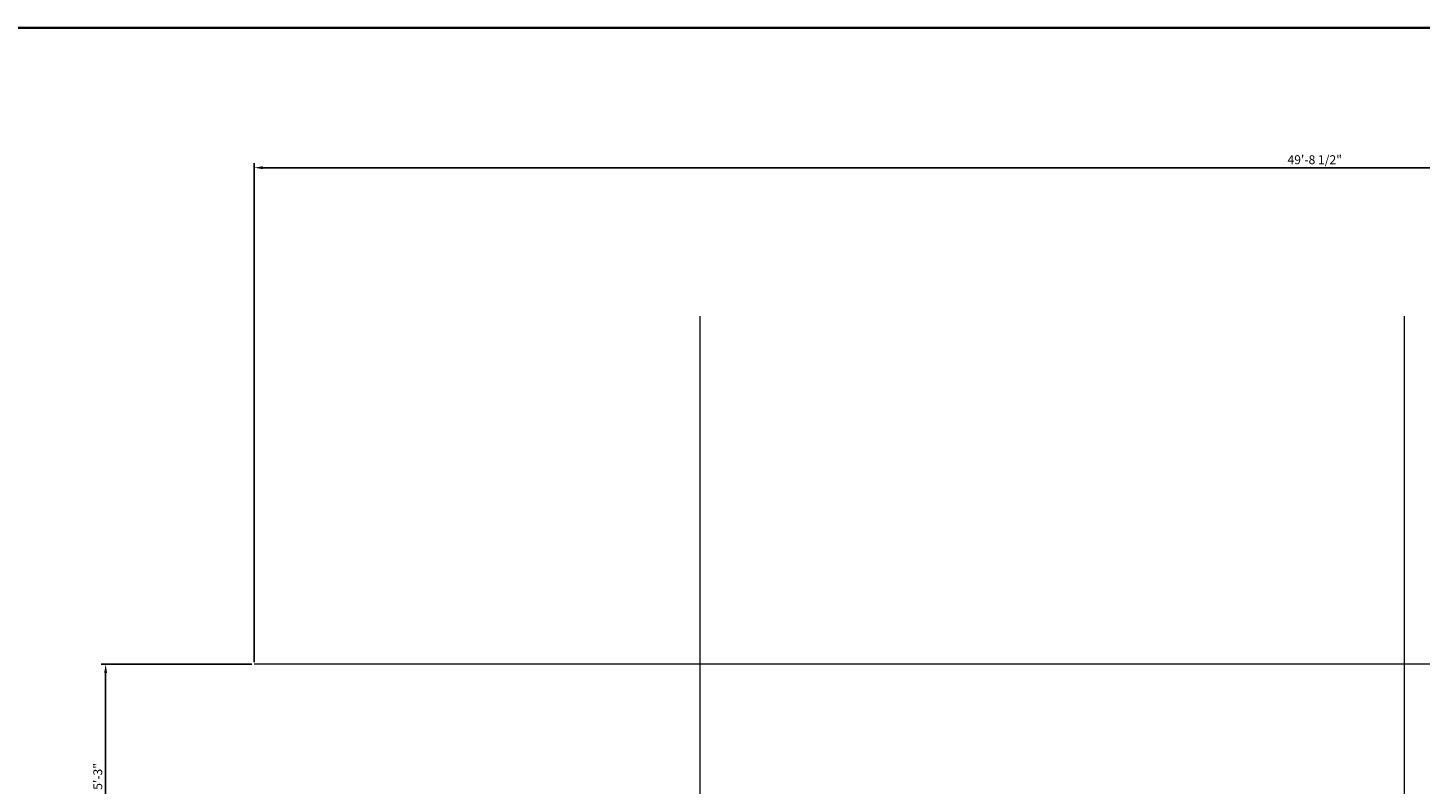
# Model space of a CAD drawing. Units: inches. Extents: x 6038 to 7543, y 3772 to 5131.
# Tile 13 of 14: x 6790 to 7182, y 4918 to 5131. Entities that reach past the tile are written whole.
import ezdxf

# ---------------------------------------------------------------- set-up
doc = ezdxf.new("R2010")
doc.units = ezdxf.units.IN
for name, color, linetype, lineweight in [('A-ANNO-DIMS', 4, 'Continuous', 18), ('A-ANNO-TTLB', 1, 'Continuous', 35), ('S-GRID', 6, 'Continuous', 13)]:
    doc.layers.add(name, color=color, linetype=linetype, lineweight=lineweight)
doc.styles.get("Standard").update_dxf_attribs({"font": 'arial.ttf'})
doc.dimstyles.new('ISO-25', dxfattribs={"dimtxt": 2.5, "dimasz": 2.5, "dimexe": 1.25, "dimexo": 0.625, "dimtad": 1, "dimdec": 0, "dimlunit": 3, "dimtxsty": 'Standard', "dimcen": 2.5, "dimadec": 0, "dimazin": 0, "dimtfac": 1, "dimtdec": 0, "dimtmove": 0, "dimatfit": 3, "dimfxl": 1, "dimarcsym": 0})

# ---------------------------------------------------------------- blocks, each defined once
blk = doc.blocks.new('*D91')
at = {"layer": 'A-ANNO-DIMS', "color": 0, "lineweight": -2, "transparency": 16777216}
for p, q in [((6853.17, 4952.12), (6810.8, 4952.12)), ((6812.05, 4891.62), (6812.05, 4949.62)), ((6853.17, 4889.12), (6810.8, 4889.12))]:
    blk.add_line(p, q, dxfattribs=at)
at = {"layer": 'A-ANNO-DIMS', "color": 0, "transparency": 16777216}
for points in [[(6811.63, 4949.62), (6812.47, 4949.62), (6812.05, 4952.12)], [(6811.63, 4891.62), (6812.47, 4891.62), (6812.05, 4889.12)]]:
    blk.add_solid(points, dxfattribs=at)
at = {"layer": 'Defpoints', "color": 0, "transparency": 16777216}
for p in [(6812.05, 4952.12), (6853.8, 4952.12), (6853.8, 4889.12)]:
    blk.add_point(p, dxfattribs=at)
at = {"layer": 'A-ANNO-DIMS', "color": 0, "transparency": 16777216, "insert": (6810.15, 4920.62), "char_height": 2.5, "attachment_point": 5, "rotation": 90}
blk.add_mtext('5\'-3"', dxfattribs=at)
blk = doc.blocks.new('*D92')
at = {"layer": 'A-ANNO-DIMS', "color": 0, "lineweight": -2, "transparency": 16777216}
for p, q in [((6853.8, 4952.74), (6853.8, 5092.84)), ((7450.09, 4952.74), (7450.09, 5092.84)), ((6856.3, 5091.59), (7447.59, 5091.59))]:
    blk.add_line(p, q, dxfattribs=at)
at = {"layer": 'A-ANNO-DIMS', "color": 0, "transparency": 16777216}
for points in [[(6856.3, 5092), (6856.3, 5091.17), (6853.8, 5091.59)], [(7447.59, 5092), (7447.59, 5091.17), (7450.09, 5091.59)]]:
    blk.add_solid(points, dxfattribs=at)
at = {"layer": 'Defpoints', "color": 0, "transparency": 16777216}
for p in [(7450.09, 5091.59), (6853.8, 4952.12), (7450.09, 4952.12)]:
    blk.add_point(p, dxfattribs=at)
at = {"layer": 'A-ANNO-DIMS', "color": 0, "transparency": 16777216, "insert": (7151.95, 5093.5), "char_height": 2.5, "attachment_point": 5}
blk.add_mtext('49\'-8 1/2"', dxfattribs=at)

msp = doc.modelspace()

# ---------------------------------------------------------------- linework, layer by layer
at = {"layer": 'A-ANNO-TTLB'}
msp.add_lwpolyline([(6037.83, 5130.86), (7542.53, 5130.86), (7542.53, 3772.09), (6037.83, 3772.09)], close=True, dxfattribs=at)
at = {"layer": 'S-GRID'}
for p, q in [((6979.09, 5049.84), (6979.09, 4893.62)), ((7177.09, 5049.84), (7177.09, 4893.62)), ((7325.59, 4952.12), (6853.8, 4952.12))]:
    msp.add_line(p, q, dxfattribs=at)

# ---------------------------------------------------------------- dimensions: what is measured, and where the dimension line sits
at = {"layer": 'A-ANNO-DIMS'}
dim = msp.add_linear_dim(base=(7450.09, 5091.59), p1=(6853.8, 4952.12), p2=(7450.09, 4952.12), dimstyle='ISO-25', override={"dimdec": 1, "dimlfac": 1, "dimrnd": 0, "dimzin": 1, "dimdsep": 46, "dimlunit": 4, "dimfrac": 2}, dxfattribs=at)
dim.commit()
dim.dimension.update_dxf_attribs({"geometry": '*D92', "text_midpoint": (7151.95, 5093.5)})
dim = msp.add_linear_dim(base=(6812.05, 4952.12), p1=(6853.8, 4889.12), p2=(6853.8, 4952.12), angle=90, dimstyle='ISO-25', override={"dimdec": 1, "dimlfac": 1, "dimrnd": 0, "dimzin": 1, "dimdsep": 46, "dimlunit": 4, "dimfrac": 2}, dxfattribs=at)
dim.commit()
dim.dimension.update_dxf_attribs({"geometry": '*D91', "text_midpoint": (6810.15, 4920.62)})

doc.saveas('drawing.dxf')
